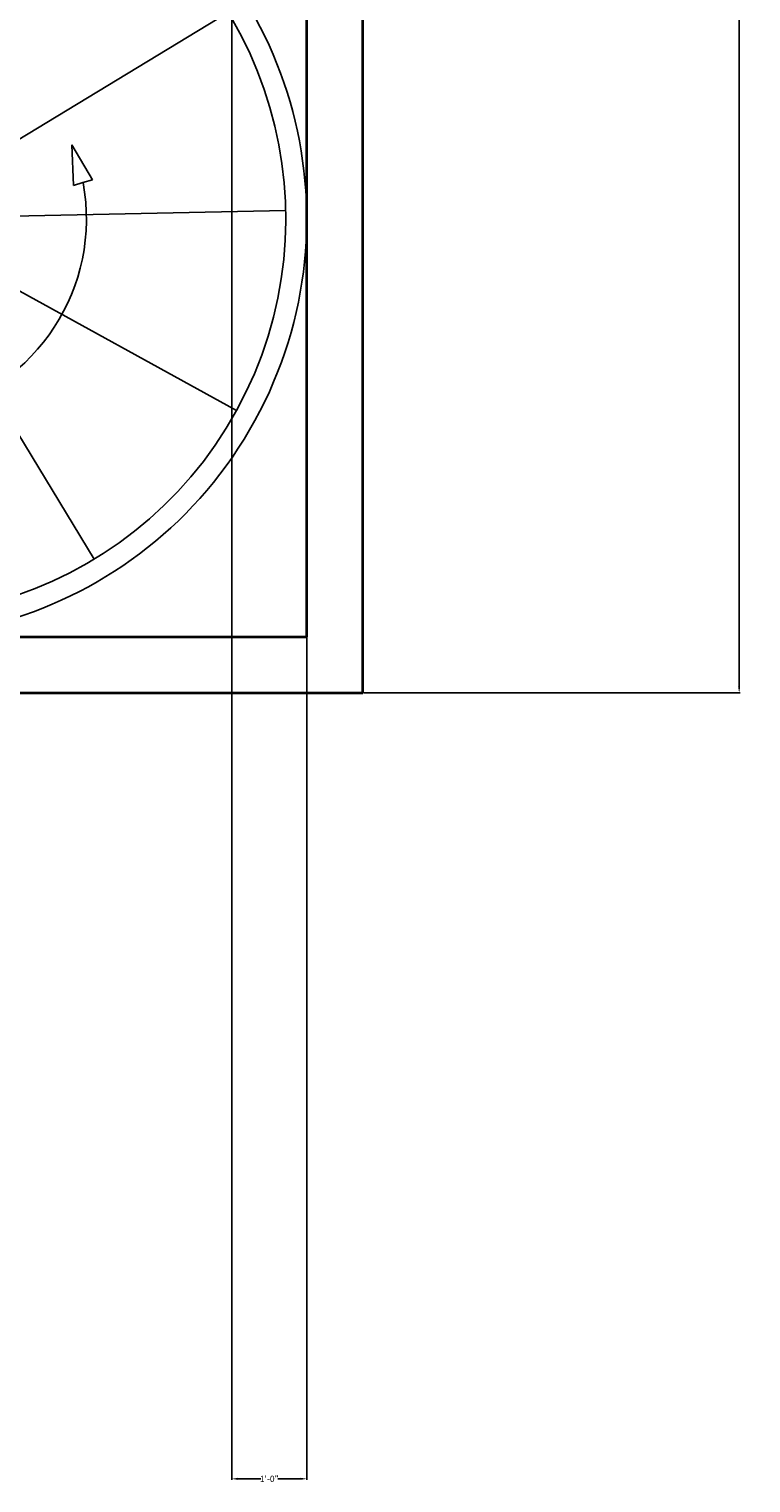
# Model space of a CAD drawing. Units: inches. Extents: x 371 to 1095, y -45 to 1219.
# Tile 4 of 18: x 979 to 1095, y -44 to 188. Entities that reach past the tile are written whole.
import ezdxf

# ---------------------------------------------------------------- set-up
doc = ezdxf.new("R2010")
doc.units = ezdxf.units.IN
doc.header["$MEASUREMENT"] = 0
for name, color, linetype, lineweight in [('A-ANNO-DIMS', 2, 'Continuous', 18), ('A-FLOR-STRS', 7, 'Continuous', 25), ('A-WALL', 40, 'Continuous', 35), ('C-SITE-WALL', 40, 'Continuous', 35)]:
    doc.layers.add(name, color=color, linetype=linetype, lineweight=lineweight)
doc.styles.get("Standard").update_dxf_attribs({"font": 'arial.ttf'})
doc.dimstyles.get("Standard").update_dxf_attribs({"dimtxt": 1, "dimasz": 1, "dimexe": 0.18, "dimexo": 0.0625, "dimgap": 0.09, "dimtad": 0, "dimtih": 1, "dimtoh": 1, "dimdec": 0, "dimzin": 0, "dimdsep": 46, "dimlunit": 3, "dimtxsty": 'Standard', "dimcen": 0.09, "dimadec": 0, "dimazin": 0, "dimtfac": 1, "dimtdec": 0, "dimtofl": 0, "dimtmove": 0, "dimatfit": 3, "dimfxl": 1, "dimtolj": 1, "dimtzin": 0, "dimarcsym": 0})

# ---------------------------------------------------------------- blocks, each defined once
blk = doc.blocks.new('Staircase - Spiral')
for p, q in [((0, 4.5), (0, 30)), ((-2.2579, 3.91), (-14.25, 24.681)), ((-3.8566, 2.226), (-24.6818, 14.25)), ((-4.5, 0), (-28.5, 0)), ((4.5, 0), (30, 0)), ((-3.8954, -2.2492), (-24.6818, -14.2502)), ((3.8999, -2.2518), (24.6817, -14.2502)), ((-2.2755, -3.9415), (-14.25, -24.6819)), ((2.2614, -3.9171), (14.25, -24.6819)), ((0, -4.5002), (0, -28.5002)), ((8.5, -10.5002), (11, -9.0002)), ((11, -9.0002), (9.5, -11.5002)), ((9, -11.0002), (8.5, -10.5002)), ((9, -11.0002), (9.5, -11.5002))]:
    blk.add_line(p, q)
blk.add_circle((0, 0), 4.5)
for radius, start, end in [(30, 90, 0), (28.5, 90, 0), (14.2215, 135, 309.2894)]:
    blk.add_arc((0, 0), radius, start, end)
blk = doc.blocks.new('*D51')
at = {"layer": 'A-ANNO-DIMS', "color": 0, "lineweight": -2, "transparency": 16777216}
for p, q in [((1032.87, 982.03), (1093.19, 982.03)), ((1093.01, 981.03), (1093.01, 532.63)), ((1093.01, 83.03), (1093.01, 531.42)), ((1032.87, 82.03), (1093.19, 82.03))]:
    blk.add_line(p, q, dxfattribs=at)
at = {"layer": 'A-ANNO-DIMS', "color": 0, "transparency": 16777216}
for points in [[(1092.84, 981.03), (1093.17, 981.03), (1093.01, 982.03)], [(1092.84, 83.03), (1093.17, 83.03), (1093.01, 82.03)]]:
    blk.add_solid(points, dxfattribs=at)
at = {"layer": 'Defpoints', "color": 0, "transparency": 16777216}
for p in [(1032.81, 982.03), (1093.01, 982.03), (1032.81, 82.03)]:
    blk.add_point(p, dxfattribs=at)
at = {"layer": 'A-ANNO-DIMS', "color": 0, "transparency": 16777216, "insert": (1093.01, 532.03), "char_height": 1, "attachment_point": 5}
blk.add_mtext('\\A1;75\'-0"', dxfattribs=at)
blk = doc.blocks.new('*D62')
at = {"layer": 'A-ANNO-DIMS', "color": 0, "lineweight": -2, "transparency": 16777216}
for p, q in [((1023.81, 450.96), (1023.81, -43.83)), ((1011.81, 441.96), (1011.81, -43.83)), ((1012.81, -43.65), (1016.44, -43.65)), ((1022.81, -43.65), (1019.18, -43.65))]:
    blk.add_line(p, q, dxfattribs=at)
at = {"layer": 'A-ANNO-DIMS', "color": 0, "transparency": 16777216}
for points in [[(1012.81, -43.48), (1012.81, -43.82), (1011.81, -43.65)], [(1022.81, -43.48), (1022.81, -43.82), (1023.81, -43.65)]]:
    blk.add_solid(points, dxfattribs=at)
at = {"layer": 'Defpoints', "color": 0, "transparency": 16777216}
for p in [(1023.81, 451.03), (1011.81, 442.03), (1023.81, -43.65)]:
    blk.add_point(p, dxfattribs=at)
at = {"layer": 'A-ANNO-DIMS', "color": 0, "transparency": 16777216, "insert": (1017.81, -43.65), "char_height": 1, "attachment_point": 5}
blk.add_mtext('\\A1;1\'-0"', dxfattribs=at)

msp = doc.modelspace()

# ---------------------------------------------------------------- linework, layer by layer
at = {"layer": 'A-WALL'}
msp.add_line((1032.81, 82.03), (1032.81, 982.03), dxfattribs=at)
at = {"layer": 'C-SITE-WALL'}
for p, q in [((1023.81, 91.03), (1023.81, 442.03)), ((828.28, 91.03), (1023.81, 91.03)), ((822.81, 82.03), (1032.81, 82.03))]:
    msp.add_line(p, q, dxfattribs=at)

# ---------------------------------------------------------------- block references
at = {"layer": 'A-FLOR-STRS', "xscale": 2.233824712970382, "yscale": 2.233824712970382, "zscale": 2.233824712970382, "rotation": 61.2124779579666}
msp.add_blockref('Staircase - Spiral', (956.78, 157.87), dxfattribs=at)

# ---------------------------------------------------------------- dimensions: what is measured, and where the dimension line sits
at = {"layer": 'A-ANNO-DIMS'}
dim = msp.add_linear_dim(base=(1093.01, 982.03), p1=(1032.81, 82.03), p2=(1032.81, 982.03), angle=90, dimstyle='Standard', override={"dimdec": 1, "dimlfac": 1, "dimrnd": 0, "dimzin": 1, "dimdsep": 46, "dimlunit": 4, "dimfrac": 2}, dxfattribs=at)
dim.commit()
dim.dimension.update_dxf_attribs({"geometry": '*D51', "text_midpoint": (1093.01, 532.03)})
dim = msp.add_linear_dim(base=(1023.81, -43.65), p1=(1011.81, 442.03), p2=(1023.81, 451.03), dimstyle='Standard', override={"dimdec": 1, "dimlfac": 1, "dimrnd": 0, "dimzin": 1, "dimdsep": 46, "dimlunit": 4, "dimfrac": 2}, dxfattribs=at)
dim.commit()
dim.dimension.update_dxf_attribs({"geometry": '*D62', "text_midpoint": (1017.81, -43.65)})

doc.saveas('drawing.dxf')
